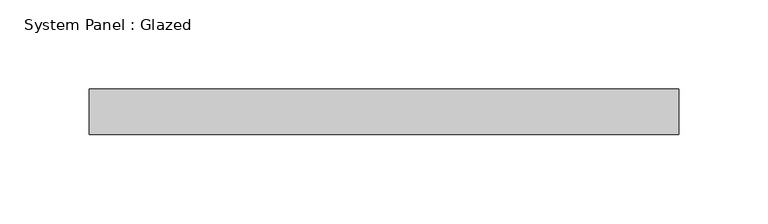
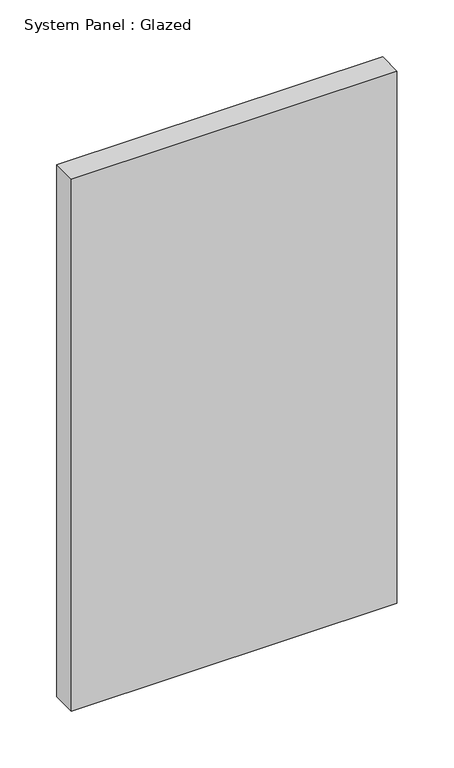
"""IFC4 building model written with IfcOpenShell, lengths in millimetres: plate geometry, System Panel : Glazed."""

from ifc_helpers import new_model, si_unit, origin, origin_with_axes, place, context, project, spatial, polyline, outline, extrude, source, transform, mapped, element, save


def system_panel_glazed_68d54f83(model_context):
    return source(origin(), model_context, "Body", "SweptSolid", [
        extrude(outline(polyline([(165.1, 19.05), (-165.1, 19.05), (-165.1, 44.45), (165.1, 44.45), (165.1, 19.05)])), origin_with_axes(), (0.0, 0.0, 1.0), 570.3342307),
    ])


if __name__ == "__main__":
    model = new_model("IFC4")
    model_context = context("Model", 3, world=origin())
    ifc_project = project(units=[si_unit("LENGTHUNIT", "METRE", prefix="MILLI")], contexts=[model_context])
    site = spatial("IfcSite", under=ifc_project)
    building = spatial("IfcBuilding", under=site)
    placement = place(None, origin())
    system_panel_glazed_shape = system_panel_glazed_68d54f83(model_context)
    element("IfcPlate", 1, ObjectType="System Panel : Glazed", at=placement, inside=building, context=model_context, shape_type="MappedRepresentation", body=[
        mapped(system_panel_glazed_shape, transform((0.0, 0.0, 0.0), x_axis=(1.0, 0.0, 0.0), y_axis=(0.0, 1.0, 0.0), z_axis=(0.0, 0.0, 1.0))),
    ])
    save(model, "model.ifc")

# Revit data of these elements
# Type "System Panel : Glazed"
#   Construction Type Id = "GSP4R"
#   Analytic Construction = "1/8 in Pilkington single glazing"
#   Visual Light Transmittance = 0.9
#   Solar Heat Gain Coefficient = 0.86
#   Heat Transfer Coefficient (U) = 1.18115 BTU/(h·ft²·°F)
#   Define Thermal Properties by = 1
# Element 1 (IfcPlate, "System Panel : Glazed")
#   Materials on its faces: "Glass"
# Materials
#   "Glass": class "Glass", colour RGB 0 128 192, transparency 0.75, Description = "Soda Lime Glass", Cost = 0
